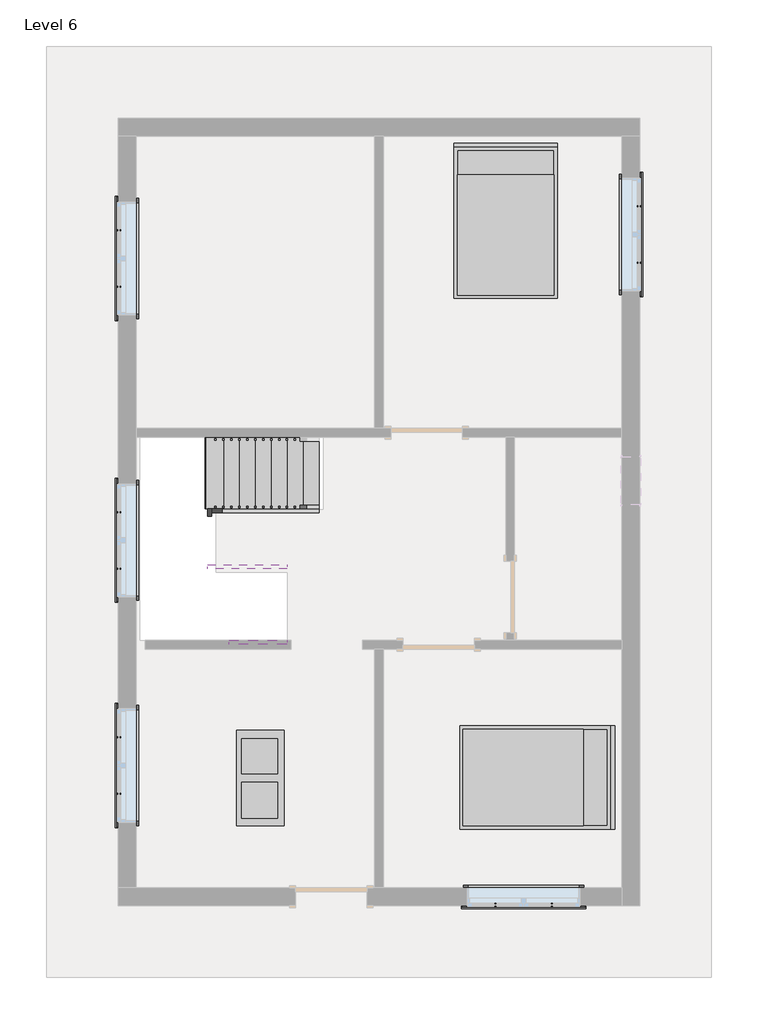
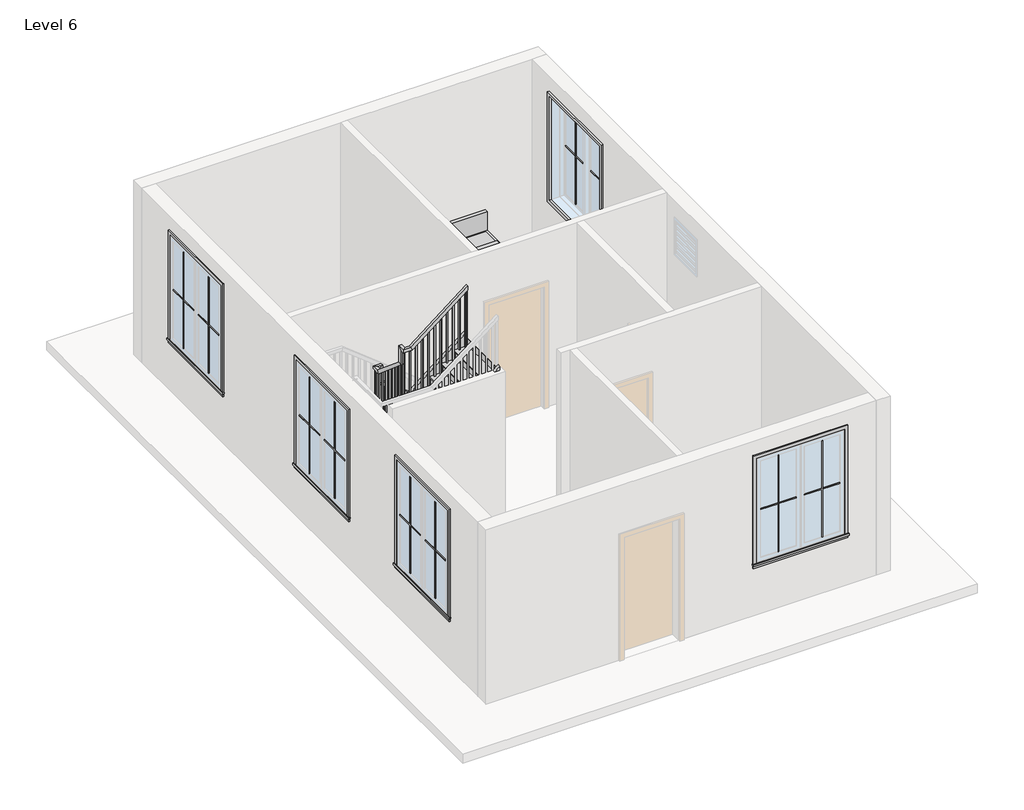
# One storey, part 2 of 2: 21 proxies, 5 members, 2 furniture elements, 1 railing, 1 stair flight.
"""IFC4 building model written with IfcOpenShell, lengths in millimetres."""

from ifc_helpers import new_model, si_unit, frame, origin, place, context, project, spatial, polyline, outline, extrude, faceted_brep, transform, mapped, element, save
from components import muntin_pattern_2x2_muntin_pattern_2x2_bff912c5, muntin_pattern_2x2_muntin_pattern_2x2_c2194282, trim_window_exterior_flat_with_sill_e04b3088, trim_window_interior_flat_picture_frame_2a7685fe, coffee_table_with_brass_mullions_11320_coffee_table_with_5962bef7, bed_17739_bed_17739_15c61121, stair_flight_d806ff93

model = new_model("IFC4")

# Units and contexts
model_context = context("Model", 3, world=origin())
ifc_project = project(units=[si_unit("LENGTHUNIT", "METRE", prefix="MILLI")], contexts=[model_context])

# Site, building, storey
site = spatial("IfcSite", under=ifc_project)
building = spatial("IfcBuilding", under=site)
storey = spatial("IfcBuildingStorey", under=building, Name="Level 6", Elevation=12801.6)

# Proxies
placement = place(None, origin())
muntin_pattern_2x2_muntin_pattern_2x2_shape = muntin_pattern_2x2_muntin_pattern_2x2_bff912c5(model_context)
element("IfcBuildingElementProxy", 1, Name="Muntin Pattern_2x2 : Muntin Pattern_2x2", ObjectType="Muntin Pattern_2x2 : Muntin Pattern_2x2", at=placement, inside=storey, context=model_context, shape_type="MappedRepresentation", body=[
    mapped(muntin_pattern_2x2_muntin_pattern_2x2_shape, transform((-626.5715247, -5050.1430046, 13785.85), x_axis=(-1.0, 0.0, 0.0), y_axis=(0.0, -1.0, 0.0), z_axis=(0.0, 0.0, 1.0))),
])
element("IfcBuildingElementProxy", 2, Name="Muntin Pattern_2x2 : Muntin Pattern_2x2", ObjectType="Muntin Pattern_2x2 : Muntin Pattern_2x2", at=placement, inside=storey, context=model_context, shape_type="MappedRepresentation", body=[
    mapped(muntin_pattern_2x2_muntin_pattern_2x2_shape, transform((-6159.0090247, -3629.3305046, 13785.85), x_axis=(0.0, 1.0, 0.0), y_axis=(-1.0, 0.0, 0.0), z_axis=(0.0, 0.0, 1.0))),
])
element("IfcBuildingElementProxy", 3, Name="Muntin Pattern_2x2 : Muntin Pattern_2x2", ObjectType="Muntin Pattern_2x2 : Muntin Pattern_2x2", at=placement, inside=storey, context=model_context, shape_type="MappedRepresentation", body=[
    mapped(muntin_pattern_2x2_muntin_pattern_2x2_shape, transform((489.4409753, 3873.1944954, 13785.85), x_axis=(0.0, -1.0, 0.0), y_axis=(1.0, 0.0, 0.0), z_axis=(0.0, 0.0, 1.0))),
])
element("IfcBuildingElementProxy", 4, Name="Muntin Pattern_2x2 : Muntin Pattern_2x2", ObjectType="Muntin Pattern_2x2 : Muntin Pattern_2x2", at=placement, inside=storey, context=model_context, shape_type="MappedRepresentation", body=[
    mapped(muntin_pattern_2x2_muntin_pattern_2x2_shape, transform((-6159.0090247, 2847.6694954, 13785.85), x_axis=(0.0, 1.0, 0.0), y_axis=(-1.0, 0.0, 0.0), z_axis=(0.0, 0.0, 1.0))),
])
element("IfcBuildingElementProxy", 5, Name="Muntin Pattern_2x2 : Muntin Pattern_2x2", ObjectType="Muntin Pattern_2x2 : Muntin Pattern_2x2", at=placement, inside=storey, context=model_context, shape_type="MappedRepresentation", body=[
    mapped(muntin_pattern_2x2_muntin_pattern_2x2_shape, transform((-6159.0090247, -752.7805046, 13785.85), x_axis=(0.0, 1.0, 0.0), y_axis=(-1.0, 0.0, 0.0), z_axis=(0.0, 0.0, 1.0))),
])
muntin_pattern_2x2_muntin_pattern_2x2_2_shape = muntin_pattern_2x2_muntin_pattern_2x2_c2194282(model_context)
element("IfcBuildingElementProxy", 6, Name="Muntin Pattern_2x2 : Muntin Pattern_2x2", ObjectType="Muntin Pattern_2x2 : Muntin Pattern_2x2", at=placement, inside=storey, context=model_context, shape_type="MappedRepresentation", body=[
    mapped(muntin_pattern_2x2_muntin_pattern_2x2_2_shape, transform((-1347.2965247, -5050.1430046, 13785.85), x_axis=(1.0, 0.0, 0.0), y_axis=(0.0, 1.0, 0.0), z_axis=(0.0, 0.0, 1.0))),
])
element("IfcBuildingElementProxy", 7, Name="Muntin Pattern_2x2 : Muntin Pattern_2x2", ObjectType="Muntin Pattern_2x2 : Muntin Pattern_2x2", at=placement, inside=storey, context=model_context, shape_type="MappedRepresentation", body=[
    mapped(muntin_pattern_2x2_muntin_pattern_2x2_2_shape, transform((-6159.0090247, -2908.6055046, 13785.85), x_axis=(0.0, -1.0, 0.0), y_axis=(1.0, 0.0, 0.0), z_axis=(0.0, 0.0, 1.0))),
])
element("IfcBuildingElementProxy", 8, Name="Muntin Pattern_2x2 : Muntin Pattern_2x2", ObjectType="Muntin Pattern_2x2 : Muntin Pattern_2x2", at=placement, inside=storey, context=model_context, shape_type="MappedRepresentation", body=[
    mapped(muntin_pattern_2x2_muntin_pattern_2x2_2_shape, transform((489.4409753, 3152.4694954, 13785.85), x_axis=(0.0, 1.0, 0.0), y_axis=(-1.0, 0.0, 0.0), z_axis=(0.0, 0.0, 1.0))),
])
element("IfcBuildingElementProxy", 9, Name="Muntin Pattern_2x2 : Muntin Pattern_2x2", ObjectType="Muntin Pattern_2x2 : Muntin Pattern_2x2", at=placement, inside=storey, context=model_context, shape_type="MappedRepresentation", body=[
    mapped(muntin_pattern_2x2_muntin_pattern_2x2_2_shape, transform((-6159.0090247, 3568.3944954, 13785.85), x_axis=(0.0, -1.0, 0.0), y_axis=(1.0, 0.0, 0.0), z_axis=(0.0, 0.0, 1.0))),
])
element("IfcBuildingElementProxy", 10, Name="Muntin Pattern_2x2 : Muntin Pattern_2x2", ObjectType="Muntin Pattern_2x2 : Muntin Pattern_2x2", at=placement, inside=storey, context=model_context, shape_type="MappedRepresentation", body=[
    mapped(muntin_pattern_2x2_muntin_pattern_2x2_2_shape, transform((-6159.0090247, -32.0555046, 13785.85), x_axis=(0.0, -1.0, 0.0), y_axis=(1.0, 0.0, 0.0), z_axis=(0.0, 0.0, 1.0))),
])
trim_window_exterior_flat_with_sill_shape = trim_window_exterior_flat_with_sill_e04b3088(model_context)
element("IfcBuildingElementProxy", 11, Name="Trim-Window-Exterior-Flat : with Sill", ObjectType="Trim-Window-Exterior-Flat : with Sill", at=placement, inside=storey, context=model_context, shape_type="MappedRepresentation", body=[
    mapped(trim_window_exterior_flat_with_sill_shape, transform((-986.9340247, -5059.6680046, 15544.8), x_axis=(1.0, 0.0, 0.0), y_axis=(0.0, 0.0, 1.0), z_axis=(0.0, -1.0, 0.0))),
])
element("IfcBuildingElementProxy", 12, Name="Trim-Window-Exterior-Flat : with Sill", ObjectType="Trim-Window-Exterior-Flat : with Sill", at=placement, inside=storey, context=model_context, shape_type="MappedRepresentation", body=[
    mapped(trim_window_exterior_flat_with_sill_shape, transform((-6168.5340247, -3268.9680046, 15544.8), x_axis=(0.0, -1.0, 0.0), y_axis=(0.0, 0.0, 1.0), z_axis=(-1.0, 0.0, 0.0))),
])
element("IfcBuildingElementProxy", 13, Name="Trim-Window-Exterior-Flat : with Sill", ObjectType="Trim-Window-Exterior-Flat : with Sill", at=placement, inside=storey, context=model_context, shape_type="MappedRepresentation", body=[
    mapped(trim_window_exterior_flat_with_sill_shape, transform((498.9659753, 3512.8319954, 15544.8), x_axis=(0.0, 1.0, 0.0), y_axis=(0.0, 0.0, 1.0), z_axis=(1.0, 0.0, 0.0))),
])
element("IfcBuildingElementProxy", 14, Name="Trim-Window-Exterior-Flat : with Sill", ObjectType="Trim-Window-Exterior-Flat : with Sill", at=placement, inside=storey, context=model_context, shape_type="MappedRepresentation", body=[
    mapped(trim_window_exterior_flat_with_sill_shape, transform((-6168.5340247, 3208.0319954, 15544.8), x_axis=(0.0, -1.0, 0.0), y_axis=(0.0, 0.0, 1.0), z_axis=(-1.0, 0.0, 0.0))),
])
element("IfcBuildingElementProxy", 15, Name="Trim-Window-Exterior-Flat : with Sill", ObjectType="Trim-Window-Exterior-Flat : with Sill", at=placement, inside=storey, context=model_context, shape_type="MappedRepresentation", body=[
    mapped(trim_window_exterior_flat_with_sill_shape, transform((-6168.5340247, -392.4180046, 15544.8), x_axis=(0.0, -1.0, 0.0), y_axis=(0.0, 0.0, 1.0), z_axis=(-1.0, 0.0, 0.0))),
])
trim_window_interior_flat_picture_frame_shape = trim_window_interior_flat_picture_frame_2a7685fe(model_context)
element("IfcBuildingElementProxy", 16, Name="Trim-Window-Interior-Flat : Picture Frame", ObjectType="Trim-Window-Interior-Flat : Picture Frame", at=placement, inside=storey, context=model_context, shape_type="MappedRepresentation", body=[
    mapped(trim_window_interior_flat_picture_frame_shape, transform((-986.9340247, -4831.0680046, 15544.8), x_axis=(-1.0, 0.0, 0.0), y_axis=(0.0, 0.0, 1.0), z_axis=(0.0, 1.0, 0.0))),
])
element("IfcBuildingElementProxy", 17, Name="Trim-Window-Interior-Flat : Picture Frame", ObjectType="Trim-Window-Interior-Flat : Picture Frame", at=placement, inside=storey, context=model_context, shape_type="MappedRepresentation", body=[
    mapped(trim_window_interior_flat_picture_frame_shape, transform((-5939.9340247, -3268.9680046, 15544.8), x_axis=(0.0, 1.0, 0.0), y_axis=(0.0, 0.0, 1.0), z_axis=(1.0, 0.0, 0.0))),
])
element("IfcBuildingElementProxy", 18, Name="Trim-Window-Interior-Flat : Picture Frame", ObjectType="Trim-Window-Interior-Flat : Picture Frame", at=placement, inside=storey, context=model_context, shape_type="MappedRepresentation", body=[
    mapped(trim_window_interior_flat_picture_frame_shape, transform((270.3659753, 3512.8319954, 15544.8), x_axis=(0.0, -1.0, 0.0), y_axis=(0.0, 0.0, 1.0), z_axis=(-1.0, 0.0, 0.0))),
])
element("IfcBuildingElementProxy", 19, Name="Trim-Window-Interior-Flat : Picture Frame", ObjectType="Trim-Window-Interior-Flat : Picture Frame", at=placement, inside=storey, context=model_context, shape_type="MappedRepresentation", body=[
    mapped(trim_window_interior_flat_picture_frame_shape, transform((-5939.9340247, 3208.0319954, 15544.8), x_axis=(0.0, 1.0, 0.0), y_axis=(0.0, 0.0, 1.0), z_axis=(1.0, 0.0, 0.0))),
])
element("IfcBuildingElementProxy", 20, Name="Trim-Window-Interior-Flat : Picture Frame", ObjectType="Trim-Window-Interior-Flat : Picture Frame", at=placement, inside=storey, context=model_context, shape_type="MappedRepresentation", body=[
    mapped(trim_window_interior_flat_picture_frame_shape, transform((-5939.9340247, -392.4180046, 15544.8), x_axis=(0.0, 1.0, 0.0), y_axis=(0.0, 0.0, 1.0), z_axis=(1.0, 0.0, 0.0))),
])
coffee_table_with_brass_mullions_11320_coffee_table_with_shape = coffee_table_with_brass_mullions_11320_coffee_table_with_5962bef7(model_context)
element("IfcBuildingElementProxy", 21, Name="coffee_table_with_brass_mullions_11320 : coffee_table_with_brass_mullions_11320", ObjectType="coffee_table_with_brass_mullions_11320 : coffee_table_with_brass_mullions_11320", at=placement, inside=storey, context=model_context, shape_type="MappedRepresentation", body=[
    mapped(coffee_table_with_brass_mullions_11320_coffee_table_with_shape, transform((-3920.6340247, -2792.7180046, 12801.6), x_axis=(0.0, 1.0, 0.0), y_axis=(-1.0, 0.0, 0.0), z_axis=(0.0, 0.0, 1.0))),
])

# Furniture
bed_17739_bed_17739_shape = bed_17739_bed_17739_15c61121(model_context)
element("IfcFurniture", 22, ObjectType="Bed_17739 : Bed_17739", at=placement, inside=storey, context=model_context, shape_type="MappedRepresentation", body=[
    mapped(bed_17739_bed_17739_shape, transform((-1215.5340247, 3665.2319954, 12801.6), x_axis=(1.0, 0.0, 0.0), y_axis=(0.0, 1.0, 0.0), z_axis=(0.0, 0.0, 1.0))),
])
element("IfcFurniture", 23, ObjectType="Bed_17739 : Bed_17739", at=placement, inside=storey, context=model_context, shape_type="MappedRepresentation", body=[
    mapped(bed_17739_bed_17739_shape, transform((-834.5340247, -3421.3680046, 12801.6), x_axis=(0.0, -1.0, 0.0), y_axis=(1.0, 0.0, 0.0), z_axis=(0.0, 0.0, 1.0))),
])

# Members
element("IfcMember", 24, ObjectType="Stringer - 2\" Width", at=placement, inside=storey, context=model_context, shape_type="SweptSolid", body=[
    extrude(outline(polyline([(12801.6, -3603.1340247), (13033.1686588, -3603.1340247), (14116.0107641, -4974.7340247), (13727.6725136, -4974.7340247), (12801.6, -3801.7088408), (12801.6, -3603.1340247)])), frame((0.0, -43.1680046, 0.0), z_axis=(0.0, 1.0, 0.0), x_axis=(0.0, 0.0, 1.0)), (0.0, 0.0, 1.0), 50.8),
])
element("IfcMember", 25, ObjectType="Stringer - 2\" Width", at=placement, inside=storey, context=model_context, shape_type="SweptSolid", body=[
    extrude(outline(polyline([(7.6319954, 14322.8930346), (7.6319954, 13924.4154064), (-703.5680046, 14523.3206696), (-703.5680046, 14921.7982978), (7.6319954, 14322.8930346)])), frame((-5025.5340247, 0.0, 0.0), z_axis=(1.0, 0.0, 0.0), x_axis=(0.0, 1.0, 0.0)), (0.0, 0.0, 1.0), 50.8),
])
element("IfcMember", 26, ObjectType="Stringer - 2\" Width", at=placement, inside=storey, context=model_context, shape_type="SweptSolid", body=[
    extrude(outline(polyline([(15118.642343, -5025.5340247), (14730.3040926, -5025.5340247), (15532.4093557, -4009.5340247), (15920.7476062, -4009.5340247), (15118.642343, -5025.5340247)])), frame((0.0, -754.3680046, 0.0), z_axis=(0.0, 1.0, 0.0), x_axis=(0.0, 0.0, 1.0)), (0.0, 0.0, 1.0), 50.8),
])
element("IfcMember", 27, ObjectType="Stringer - 2\" Width", at=placement, inside=storey, context=model_context, shape_type="SweptSolid", body=[
    extrude(outline(polyline([(12801.6, -3603.1340247), (13033.1686588, -3603.1340247), (13552.871982, -4261.4249007), (13552.871982, -4753.3200179), (12801.6, -3801.7088408), (12801.6, -3603.1340247)])), frame((0.0, 922.0319954, 0.0), z_axis=(0.0, 1.0, 0.0), x_axis=(0.0, 0.0, 1.0)), (0.0, 0.0, 1.0), 50.8),
])
element("IfcMember", 28, ObjectType="Stringer - 2\" Width", at=placement, inside=storey, context=model_context, shape_type="SweptSolid", body=[
    extrude(outline(polyline([(15336.1206696, -4258.1663605), (15532.4093557, -4009.5340247), (15920.7476062, -4009.5340247), (15336.1206696, -4750.0614777), (15336.1206696, -4258.1663605)])), frame((0.0, -1719.5680046, 0.0), z_axis=(0.0, 1.0, 0.0), x_axis=(0.0, 0.0, 1.0)), (0.0, 0.0, 1.0), 50.8),
])

# Railing
element("IfcRailing", 29, ObjectType="Handrail - Rectangular", at=placement, inside=storey, context=model_context, shape_type="SolidModel", body=[
    faceted_brep([(-3603.1340247, 7.6319954, 13876.4210526), (-3603.1340247, 7.6319954, 13811.6980109), (-3603.1340247, 58.4319954, 13811.6980109), (-3603.1340247, 58.4319954, 13876.4210526), (-4949.3340247, 7.6319954, 14939.2105263), (-5000.1340247, 7.6319954, 14914.5927477), (-5000.1340247, 58.4319954, 14914.5927477), (-4949.3340247, 58.4319954, 14939.2105263), (-4949.3340247, 7.6319954, 15223.9578947), (-5000.1340247, 7.6319954, 15173.1578947), (-5000.1340247, 58.4319954, 15173.1578947), (-4949.3340247, 58.4319954, 15223.9578947), (-5025.5340247, 7.6319954, 15223.9578947), (-5025.5340247, 7.6319954, 15173.1578947), (-5076.3340247, 58.4319954, 15173.1578947), (-5076.3340247, 58.4319954, 15223.9578947), (-5025.5340247, -68.5680046, 15223.9578947), (-5025.5340247, -87.1083685, 15173.1578947), (-5076.3340247, -87.1083685, 15173.1578947), (-5076.3340247, -68.5680046, 15223.9578947), (-5025.5340247, -678.1680046, 15737.3052632), (-5025.5340247, -728.9680046, 15713.6712725), (-5076.3340247, -728.9680046, 15713.6712725), (-5076.3340247, -678.1680046, 15737.3052632), (-5025.5340247, -678.1680046, 16022.0526316), (-5025.5340247, -728.9680046, 15971.2526316), (-5076.3340247, -728.9680046, 15971.2526316), (-5076.3340247, -678.1680046, 16022.0526316), (-5025.5340247, -754.3680046, 16022.0526316), (-5025.5340247, -754.3680046, 15971.2526316), (-5076.3340247, -805.1680046, 15971.2526316), (-5076.3340247, -805.1680046, 16022.0526316), (-4949.3340247, -754.3680046, 16022.0526316), (-4931.6981718, -754.3680046, 15971.2526316), (-4931.6981718, -805.1680046, 15971.2526316), (-4949.3340247, -805.1680046, 16022.0526316), (-4009.5340247, -754.3680046, 16764.0), (-4009.5340247, -805.1680046, 16764.0), (-4009.5340247, -805.1680046, 16699.2769583), (-4009.5340247, -754.3680046, 16699.2769583)], [[[0, 1, 2, 3]], [[1, 0, 4, 5]], [[2, 1, 5, 6]], [[3, 2, 6, 7]], [[0, 3, 7, 4]], [[5, 4, 8, 9]], [[6, 5, 9, 10]], [[7, 6, 10, 11]], [[4, 7, 11, 8]], [[9, 8, 12, 13]], [[10, 9, 13, 14]], [[11, 10, 14, 15]], [[8, 11, 15, 12]], [[13, 12, 16, 17]], [[14, 13, 17, 18]], [[15, 14, 18, 19]], [[12, 15, 19, 16]], [[17, 16, 20, 21]], [[18, 17, 21, 22]], [[19, 18, 22, 23]], [[16, 19, 23, 20]], [[21, 20, 24, 25]], [[22, 21, 25, 26]], [[23, 22, 26, 27]], [[20, 23, 27, 24]], [[25, 24, 28, 29]], [[26, 25, 29, 30]], [[27, 26, 30, 31]], [[24, 27, 31, 28]], [[29, 28, 32, 33]], [[30, 29, 33, 34]], [[31, 30, 34, 35]], [[28, 31, 35, 32]], [[36, 37, 38, 39]], [[33, 32, 36, 39]], [[34, 33, 39, 38]], [[35, 34, 38, 37]], [[32, 35, 37, 36]]]),
    extrude(outline(polyline([(16671.7045898, -4044.4590247), (15689.1789474, -4044.4590247), (15689.1789474, -4025.4090247), (16686.7440635, -4025.4090247), (16671.7045898, -4044.4590247)])), frame((0.0, -789.2930046, 0.0), z_axis=(0.0, 1.0, 0.0), x_axis=(0.0, 0.0, 1.0)), (0.0, 0.0, 1.0), 19.05),
    extrude(outline(polyline([(16591.4940635, -4146.0590247), (15689.1789474, -4146.0590247), (15689.1789474, -4127.0090247), (16606.5335372, -4127.0090247), (16591.4940635, -4146.0590247)])), frame((0.0, -789.2930046, 0.0), z_axis=(0.0, 1.0, 0.0), x_axis=(0.0, 0.0, 1.0)), (0.0, 0.0, 1.0), 19.05),
    extrude(outline(polyline([(16511.2835372, -4247.6590247), (15528.7578947, -4247.6590247), (15528.7578947, -4228.6090247), (16526.3230109, -4228.6090247), (16511.2835372, -4247.6590247)])), frame((0.0, -789.2930046, 0.0), z_axis=(0.0, 1.0, 0.0), x_axis=(0.0, 0.0, 1.0)), (0.0, 0.0, 1.0), 19.05),
    extrude(outline(polyline([(16431.0730109, -4349.2590247), (15528.7578947, -4349.2590247), (15528.7578947, -4330.2090247), (16446.1124846, -4330.2090247), (16431.0730109, -4349.2590247)])), frame((0.0, -789.2930046, 0.0), z_axis=(0.0, 1.0, 0.0), x_axis=(0.0, 0.0, 1.0)), (0.0, 0.0, 1.0), 19.05),
    extrude(outline(polyline([(16350.8624846, -4450.8590247), (15368.3368421, -4450.8590247), (15368.3368421, -4431.8090247), (16365.9019583, -4431.8090247), (16350.8624846, -4450.8590247)])), frame((0.0, -789.2930046, 0.0), z_axis=(0.0, 1.0, 0.0), x_axis=(0.0, 0.0, 1.0)), (0.0, 0.0, 1.0), 19.05),
    extrude(outline(polyline([(16270.6519583, -4552.4590247), (15368.3368421, -4552.4590247), (15368.3368421, -4533.4090247), (16285.6914319, -4533.4090247), (16270.6519583, -4552.4590247)])), frame((0.0, -789.2930046, 0.0), z_axis=(0.0, 1.0, 0.0), x_axis=(0.0, 0.0, 1.0)), (0.0, 0.0, 1.0), 19.05),
    extrude(outline(polyline([(16190.4414319, -4654.0590247), (15207.9157895, -4654.0590247), (15207.9157895, -4635.0090247), (16205.4809056, -4635.0090247), (16190.4414319, -4654.0590247)])), frame((0.0, -789.2930046, 0.0), z_axis=(0.0, 1.0, 0.0), x_axis=(0.0, 0.0, 1.0)), (0.0, 0.0, 1.0), 19.05),
    extrude(outline(polyline([(16110.2309056, -4755.6590247), (15207.9157895, -4755.6590247), (15207.9157895, -4736.6090247), (16125.2703793, -4736.6090247), (16110.2309056, -4755.6590247)])), frame((0.0, -789.2930046, 0.0), z_axis=(0.0, 1.0, 0.0), x_axis=(0.0, 0.0, 1.0)), (0.0, 0.0, 1.0), 19.05),
    extrude(outline(polyline([(16030.0203793, -4857.2590247), (15047.4947368, -4857.2590247), (15047.4947368, -4838.2090247), (16045.059853, -4838.2090247), (16030.0203793, -4857.2590247)])), frame((0.0, -789.2930046, 0.0), z_axis=(0.0, 1.0, 0.0), x_axis=(0.0, 0.0, 1.0)), (0.0, 0.0, 1.0), 19.05),
    extrude(outline(polyline([(15949.809853, -4958.8590247), (15047.4947368, -4958.8590247), (15047.4947368, -4939.8090247), (15964.8493267, -4939.8090247), (15949.809853, -4958.8590247)])), frame((0.0, -789.2930046, 0.0), z_axis=(0.0, 1.0, 0.0), x_axis=(0.0, 0.0, 1.0)), (0.0, 0.0, 1.0), 19.05),
    extrude(outline(polyline([(-668.6430046, 15662.8712725), (-668.6430046, 14726.6526316), (-687.6930046, 14726.6526316), (-687.6930046, 15678.9133778), (-668.6430046, 15662.8712725)])), frame((-5060.4590247, 0.0, 0.0), z_axis=(1.0, 0.0, 0.0), x_axis=(0.0, 1.0, 0.0)), (0.0, 0.0, 1.0), 19.05),
    extrude(outline(polyline([(-567.0430046, 15577.3133778), (-567.0430046, 14726.6526316), (-586.0930046, 14726.6526316), (-586.0930046, 15593.355483), (-567.0430046, 15577.3133778)])), frame((-5060.4590247, 0.0, 0.0), z_axis=(1.0, 0.0, 0.0), x_axis=(0.0, 1.0, 0.0)), (0.0, 0.0, 1.0), 19.05),
    extrude(outline(polyline([(-465.4430046, 15491.755483), (-465.4430046, 14566.2315789), (-484.4930046, 14566.2315789), (-484.4930046, 15507.7975883), (-465.4430046, 15491.755483)])), frame((-5060.4590247, 0.0, 0.0), z_axis=(1.0, 0.0, 0.0), x_axis=(0.0, 1.0, 0.0)), (0.0, 0.0, 1.0), 19.05),
    extrude(outline(polyline([(-363.8430046, 15406.1975883), (-363.8430046, 14566.2315789), (-382.8930046, 14566.2315789), (-382.8930046, 15422.2396935), (-363.8430046, 15406.1975883)])), frame((-5060.4590247, 0.0, 0.0), z_axis=(1.0, 0.0, 0.0), x_axis=(0.0, 1.0, 0.0)), (0.0, 0.0, 1.0), 19.05),
    extrude(outline(polyline([(-262.2430046, 15320.6396935), (-262.2430046, 14405.8105263), (-281.2930046, 14405.8105263), (-281.2930046, 15336.6817988), (-262.2430046, 15320.6396935)])), frame((-5060.4590247, 0.0, 0.0), z_axis=(1.0, 0.0, 0.0), x_axis=(0.0, 1.0, 0.0)), (0.0, 0.0, 1.0), 19.05),
    extrude(outline(polyline([(-160.6430046, 15235.0817988), (-160.6430046, 14405.8105263), (-179.6930046, 14405.8105263), (-179.6930046, 15251.1239041), (-160.6430046, 15235.0817988)])), frame((-5060.4590247, 0.0, 0.0), z_axis=(1.0, 0.0, 0.0), x_axis=(0.0, 1.0, 0.0)), (0.0, 0.0, 1.0), 19.05),
    extrude(outline(polyline([(-59.0430046, 15149.5239041), (-59.0430046, 14245.3894737), (-78.0930046, 14245.3894737), (-78.0930046, 15165.5660093), (-59.0430046, 15149.5239041)])), frame((-5060.4590247, 0.0, 0.0), z_axis=(1.0, 0.0, 0.0), x_axis=(0.0, 1.0, 0.0)), (0.0, 0.0, 1.0), 19.05),
    extrude(outline(polyline([(-5016.0090247, 23.5069954), (-5035.0590247, 23.5069954), (-5035.0590247, 42.5569954), (-5016.0090247, 42.5569954), (-5016.0090247, 23.5069954)])), frame((0.0, 0.0, 14084.9684211), z_axis=(0.0, 0.0, 1.0), x_axis=(1.0, 0.0, 0.0)), (0.0, 0.0, 1.0), 1088.1894737),
    extrude(outline(polyline([(14861.9545898, -4933.4590247), (13924.5473684, -4933.4590247), (13924.5473684, -4914.4090247), (14846.9151161, -4914.4090247), (14861.9545898, -4933.4590247)])), frame((0.0, 23.5069954, 0.0), z_axis=(0.0, 1.0, 0.0), x_axis=(0.0, 0.0, 1.0)), (0.0, 0.0, 1.0), 19.05),
    extrude(outline(polyline([(14781.7440635, -4831.8590247), (13924.5473684, -4831.8590247), (13924.5473684, -4812.8090247), (14766.7045898, -4812.8090247), (14781.7440635, -4831.8590247)])), frame((0.0, 23.5069954, 0.0), z_axis=(0.0, 1.0, 0.0), x_axis=(0.0, 0.0, 1.0)), (0.0, 0.0, 1.0), 19.05),
    extrude(outline(polyline([(14701.5335372, -4730.2590247), (13764.1263158, -4730.2590247), (13764.1263158, -4711.2090247), (14686.4940635, -4711.2090247), (14701.5335372, -4730.2590247)])), frame((0.0, 23.5069954, 0.0), z_axis=(0.0, 1.0, 0.0), x_axis=(0.0, 0.0, 1.0)), (0.0, 0.0, 1.0), 19.05),
    extrude(outline(polyline([(14621.3230109, -4628.6590247), (13764.1263158, -4628.6590247), (13764.1263158, -4609.6090247), (14606.2835372, -4609.6090247), (14621.3230109, -4628.6590247)])), frame((0.0, 23.5069954, 0.0), z_axis=(0.0, 1.0, 0.0), x_axis=(0.0, 0.0, 1.0)), (0.0, 0.0, 1.0), 19.05),
    extrude(outline(polyline([(14541.1124846, -4527.0590247), (13603.7052632, -4527.0590247), (13603.7052632, -4508.0090247), (14526.0730109, -4508.0090247), (14541.1124846, -4527.0590247)])), frame((0.0, 23.5069954, 0.0), z_axis=(0.0, 1.0, 0.0), x_axis=(0.0, 0.0, 1.0)), (0.0, 0.0, 1.0), 19.05),
    extrude(outline(polyline([(14460.9019583, -4425.4590247), (13603.7052632, -4425.4590247), (13603.7052632, -4406.4090247), (14445.8624846, -4406.4090247), (14460.9019583, -4425.4590247)])), frame((0.0, 23.5069954, 0.0), z_axis=(0.0, 1.0, 0.0), x_axis=(0.0, 0.0, 1.0)), (0.0, 0.0, 1.0), 19.05),
    extrude(outline(polyline([(14380.6914319, -4323.8590247), (13443.2842105, -4323.8590247), (13443.2842105, -4304.8090247), (14365.6519583, -4304.8090247), (14380.6914319, -4323.8590247)])), frame((0.0, 23.5069954, 0.0), z_axis=(0.0, 1.0, 0.0), x_axis=(0.0, 0.0, 1.0)), (0.0, 0.0, 1.0), 19.05),
    extrude(outline(polyline([(14300.4809056, -4222.2590247), (13443.2842105, -4222.2590247), (13443.2842105, -4203.2090247), (14285.4414319, -4203.2090247), (14300.4809056, -4222.2590247)])), frame((0.0, 23.5069954, 0.0), z_axis=(0.0, 1.0, 0.0), x_axis=(0.0, 0.0, 1.0)), (0.0, 0.0, 1.0), 19.05),
    extrude(outline(polyline([(14220.2703793, -4120.6590247), (13282.8631579, -4120.6590247), (13282.8631579, -4101.6090247), (14205.2309056, -4101.6090247), (14220.2703793, -4120.6590247)])), frame((0.0, 23.5069954, 0.0), z_axis=(0.0, 1.0, 0.0), x_axis=(0.0, 0.0, 1.0)), (0.0, 0.0, 1.0), 19.05),
    extrude(outline(polyline([(14140.059853, -4019.0590247), (13282.8631579, -4019.0590247), (13282.8631579, -4000.0090247), (14125.0203793, -4000.0090247), (14140.059853, -4019.0590247)])), frame((0.0, 23.5069954, 0.0), z_axis=(0.0, 1.0, 0.0), x_axis=(0.0, 0.0, 1.0)), (0.0, 0.0, 1.0), 19.05),
    extrude(outline(polyline([(14059.8493267, -3917.4590247), (13122.4421053, -3917.4590247), (13122.4421053, -3898.4090247), (14044.809853, -3898.4090247), (14059.8493267, -3917.4590247)])), frame((0.0, 23.5069954, 0.0), z_axis=(0.0, 1.0, 0.0), x_axis=(0.0, 0.0, 1.0)), (0.0, 0.0, 1.0), 19.05),
    extrude(outline(polyline([(13979.6388004, -3815.8590247), (13122.4421053, -3815.8590247), (13122.4421053, -3796.8090247), (13964.5993267, -3796.8090247), (13979.6388004, -3815.8590247)])), frame((0.0, 23.5069954, 0.0), z_axis=(0.0, 1.0, 0.0), x_axis=(0.0, 0.0, 1.0)), (0.0, 0.0, 1.0), 19.05),
    extrude(outline(polyline([(13899.428274, -3714.2590247), (12962.0210526, -3714.2590247), (12962.0210526, -3695.2090247), (13884.3888004, -3695.2090247), (13899.428274, -3714.2590247)])), frame((0.0, 23.5069954, 0.0), z_axis=(0.0, 1.0, 0.0), x_axis=(0.0, 0.0, 1.0)), (0.0, 0.0, 1.0), 19.05),
    extrude(outline(polyline([(-5041.4090247, -770.2430046), (-5041.4090247, -789.2930046), (-5060.4590247, -789.2930046), (-5060.4590247, -770.2430046), (-5041.4090247, -770.2430046)])), frame((0.0, 0.0, 14887.0736842), z_axis=(0.0, 0.0, 1.0), x_axis=(1.0, 0.0, 0.0)), (0.0, 0.0, 1.0), 1084.1789474),
    extrude(outline(polyline([(-5041.4090247, 23.5069954), (-5060.4590247, 23.5069954), (-5060.4590247, 42.5569954), (-5041.4090247, 42.5569954), (-5041.4090247, 23.5069954)])), frame((0.0, 0.0, 14084.9684211), z_axis=(0.0, 0.0, 1.0), x_axis=(1.0, 0.0, 0.0)), (0.0, 0.0, 1.0), 1088.1894737),
    extrude(outline(polyline([(16684.2374846, -4028.5840247), (15689.1789474, -4028.5840247), (15689.1789474, -4009.5340247), (16699.2769583, -4009.5340247), (16684.2374846, -4028.5840247)])), frame((0.0, -789.2930046, 0.0), z_axis=(0.0, 1.0, 0.0), x_axis=(0.0, 0.0, 1.0)), (0.0, 0.0, 1.0), 19.05),
    extrude(outline(polyline([(13826.7374846, -3622.1840247), (12962.0210526, -3622.1840247), (12962.0210526, -3603.1340247), (13811.6980109, -3603.1340247), (13826.7374846, -3622.1840247)])), frame((0.0, 23.5069954, 0.0), z_axis=(0.0, 1.0, 0.0), x_axis=(0.0, 0.0, 1.0)), (0.0, 0.0, 1.0), 19.05),
])

# Stair flight
stair_flight_shape = stair_flight_d806ff93(model_context)
element("IfcStairFlight", 30, ObjectType="2\" Tread 1\" Nosing 1/4\" Riser", at=placement, inside=storey, context=model_context, shape_type="MappedRepresentation", body=[
    mapped(stair_flight_shape, transform((0.0, 0.0, 0.0), x_axis=(1.0, 0.0, 0.0), y_axis=(0.0, 1.0, 0.0), z_axis=(0.0, 0.0, 1.0))),
])

save(model, "model.ifc")

# Revit data of these elements
# Type "Muntin Pattern_2x2 : Muntin Pattern_2x2"
#   Width [instance default] = 4' - 0"
#   Thickness = 0' - 0 1/2"
#   Height [instance default] = 4' - 0"
#   Distance = 0' - 0 3/4"
#   Interior Material [instance default] = none
#   Exterior Material [instance default] = none
#   Default Elevation = 0
# Type "Trim-Window-Exterior-Flat : with Sill"
#   Trim Width = 0' - 2 1/4"
#   Trim Thickness_Picture Frame = 0' - 1 1/4"
#   Trim Thickness_with Sill = 0' - 0 3/4"
#   Sill Thickness = 0' - 1 1/4"
#   Opening Width [instance default] = 2' - 0"
#   Opening Height [instance default] = 3' - 0"
#   Default Elevation = 4' - 0"
#   Sill = yes
#   Picture Frame = no
#   Trim Material [instance default] = none
# Type "Trim-Window-Interior-Flat : Picture Frame"
#   Trim Thickness_Picture Frame = 0' - 1 1/4"
#   Trim Width = 0' - 2 1/4"
#   Trim Thickness_with Sill = 0' - 0 3/4"
#   Sill Thickness = 0' - 1 1/4"
#   Opening Width [instance default] = 2' - 0"
#   Opening Height [instance default] = 3' - 0"
#   Default Elevation = 4' - 0"
#   Sill = no
#   Picture Frame = yes
#   Trim Material [instance default] = none
# Type "coffee_table_with_brass_mullions_11320 : coffee_table_with_brass_mullions_11320"
#   Default Elevation = 0
# Type "Bed_17739 : Bed_17739"
#   Default Elevation = 0
# Type "Handrail - Rectangular"
#   Assembly Code = "C2010400"
#   built-in parameter 1008612 = 0.0416667 (stored number, unit not read)
#   built-in parameter 1008611 = 0.0416667 (stored number, unit not read)
#   built-in parameter 1008609 = 0.333333 (stored number, unit not read)
#   built-in parameter 1008604 = 0.166667 (stored number, unit not read)
#   built-in parameter 1008603 = 0.166667 (stored number, unit not read)
#   Railing Height = 3' - 0"
#   built-in parameter 1008630 = 2
#   built-in parameter 1008610 = 2
#   built-in parameter 1008618 = Baluster - Square : 3/4"
# Elements 1, 2, 3, 4, 5, 6, 7, 8, 9, 10 (IfcBuildingElementProxy, "Muntin Pattern_2x2 : Muntin Pattern_2x2")
#   Width = 1' - 11 1/8"
#   Height = 5' - 6 1/2"
#   Interior Material = Wood - Stained
#   Exterior Material = Clad - White
#   Phase Created = New Construction
#   Materials on its faces: "Clad - White", "Wood - Stained"
# Elements 11, 12, 13, 14, 15 (IfcBuildingElementProxy, "Trim-Window-Exterior-Flat : with Sill")
#   Opening Width = 4' - 9"
#   Opening Height = 6' - 0"
#   Trim Material = Clad - White
#   Phase Created = New Construction
#   Materials on its faces: "Clad - White"
# Elements 16, 17, 18, 19, 20 (IfcBuildingElementProxy, "Trim-Window-Interior-Flat : Picture Frame")
#   Opening Width = 4' - 9"
#   Opening Height = 6' - 0"
#   Trim Material = Wood - Stained
#   Phase Created = New Construction
#   Materials on its faces: "Wood - Stained"
# Element 21 (IfcBuildingElementProxy, "coffee_table_with_brass_mullions_11320 : coffee_table_with_brass_mullions_11320")
#   Phase Created = New Construction
#   Materials on its faces: "Default Wall", "TABLE", "Glass", "Default"
# Elements 22, 23 (IfcFurniture, "Bed_17739 : Bed_17739")
#   Phase Created = New Construction
#   Materials on its faces: "legs", "sheets", "bed frame", "Blanket"
# Elements 24, 25, 26, 27, 28 (IfcMember, "Stringer - 2\" Width")
#   Phase Created = New Construction
# Element 29 (IfcRailing, "Handrail - Rectangular")
#   Phase Created = New Construction
#   Materials on its faces: "Oak Flooring"
# Element 30 (IfcStairFlight, "2\" Tread 1\" Nosing 1/4\" Riser")
#   Phase Created = New Construction
# Materials
#   "Clad - White": class "Wood", colour RGB 242 242 238, transparency 0, Cost = 0
#   "Wood - Stained": class "Wood", colour RGB 224 178 126, transparency 0, Cost = 0
#   "Default Wall": colour RGB 128 128 128, transparency 0, Cost = 0
#   "TABLE": class "Generic", colour RGB 120 120 120, transparency 0, Cost = 0
#   "Glass": class "Glass", colour RGB 0 128 192, transparency 0.75, Description = "Soda Lime Glass", Cost = 0
#   "Default": colour RGB 127 127 127, transparency 0, Cost = 0
#   "legs": colour RGB 90 73 37, transparency 0, Cost = 0
#   "sheets": colour RGB 200 195 176, transparency 0, Cost = 0
#   "bed frame": colour RGB 90 73 37, transparency 0, Cost = 0
#   "Blanket": class "System", colour RGB 59 0 1, transparency 0, Cost = 0
#   "Oak Flooring": class "Wood", colour RGB 216 169 114, transparency 0, Description = "Quercus Rubra", Cost = 0
